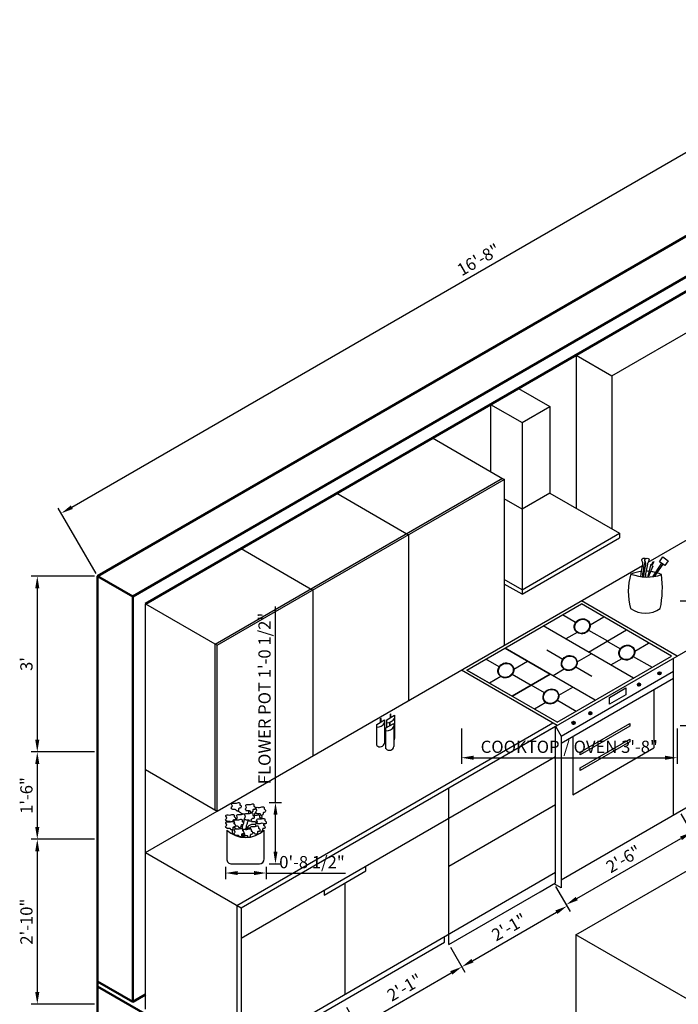
# Model space of a CAD drawing. Units: inches. Extents: x 5770 to 11891, y 3254 to 6808.
# Tile 2 of 15: x 5770 to 5905, y 3361 to 3563. Entities that reach past the tile are written whole.
import ezdxf

# ---------------------------------------------------------------- set-up
doc = ezdxf.new("R2010")
doc.units = ezdxf.units.IN
for name, color, linetype, lineweight in [('A-ANNO-DIMS', 2, 'Continuous', 18), ('A-ANNO-SYMB', 7, 'Continuous', 18), ('A-EQPM', 6, 'Continuous', 25), ('A-FURN', 8, 'Continuous', 25), ('A-WALL', 7, 'Continuous', 50)]:
    doc.layers.add(name, color=color, linetype=linetype, lineweight=lineweight)
doc.styles.get("Standard").update_dxf_attribs({"font": 'arial.ttf'})
doc.dimstyles.new('ISO-25', dxfattribs={"dimtxt": 2.5, "dimasz": 2.5, "dimexe": 1.25, "dimexo": 0.625, "dimtad": 1, "dimdec": 0, "dimlunit": 3, "dimtxsty": 'Standard', "dimcen": 2.5, "dimadec": 0, "dimazin": 0, "dimtfac": 1, "dimtdec": 0, "dimtmove": 0, "dimatfit": 3, "dimfxl": 1, "dimarcsym": 0})

# ---------------------------------------------------------------- blocks, each defined once
blk = doc.blocks.new('*D2')
at = {"layer": 'A-ANNO-DIMS', "color": 0, "lineweight": -2, "transparency": 16777216}
for p, q in [((5858.42, 3372.87), (5861.37, 3367.75)), ((5841.62, 3357.79), (5858.58, 3367.59)), ((5837.13, 3360.58), (5840.08, 3355.46))]:
    blk.add_line(p, q, dxfattribs=at)
at = {"layer": 'A-ANNO-DIMS', "color": 0, "transparency": 16777216}
for points in [[(5858.37, 3367.95), (5858.79, 3367.23), (5860.75, 3368.84)], [(5841.41, 3358.15), (5841.83, 3357.43), (5839.46, 3356.54)]]:
    blk.add_solid(points, dxfattribs=at)
at = {"layer": 'Defpoints', "color": 0, "transparency": 16777216}
for p in [(5858.1, 3373.41), (5860.75, 3368.84), (5836.81, 3361.12)]:
    blk.add_point(p, dxfattribs=at)
at = {"layer": 'A-ANNO-DIMS', "color": 0, "transparency": 16777216, "insert": (5849.16, 3364.32), "char_height": 2.5, "attachment_point": 5, "rotation": 30}
blk.add_mtext('2\'-1"', dxfattribs=at)
blk = doc.blocks.new('*D3')
at = {"layer": 'A-ANNO-DIMS', "color": 0, "lineweight": -2, "transparency": 16777216}
for p, q in [((5879.96, 3385.31), (5882.91, 3380.19)), ((5862.91, 3370.09), (5880.12, 3380.02)), ((5858.42, 3372.87), (5861.37, 3367.75))]:
    blk.add_line(p, q, dxfattribs=at)
at = {"layer": 'A-ANNO-DIMS', "color": 0, "transparency": 16777216}
for points in [[(5879.91, 3380.38), (5880.33, 3379.66), (5882.29, 3381.27)], [(5862.7, 3370.45), (5863.12, 3369.73), (5860.75, 3368.84)]]:
    blk.add_solid(points, dxfattribs=at)
at = {"layer": 'Defpoints', "color": 0, "transparency": 16777216}
for p in [(5879.65, 3385.85), (5882.29, 3381.27), (5858.1, 3373.41)]:
    blk.add_point(p, dxfattribs=at)
at = {"layer": 'A-ANNO-DIMS', "color": 0, "transparency": 16777216, "insert": (5870.58, 3376.68), "char_height": 2.5, "attachment_point": 5, "rotation": 30}
blk.add_mtext('2\'-1"', dxfattribs=at)
blk = doc.blocks.new('*D4')
at = {"layer": 'A-ANNO-DIMS', "color": 0, "lineweight": -2, "transparency": 16777216}
for p, q in [((5905.64, 3400.14), (5908.43, 3395.3)), ((5884.29, 3382.81), (5905.64, 3395.14)), ((5879.96, 3385.31), (5882.75, 3380.47))]:
    blk.add_line(p, q, dxfattribs=at)
at = {"layer": 'A-ANNO-DIMS', "color": 0, "transparency": 16777216}
for points in [[(5905.43, 3395.5), (5905.85, 3394.77), (5907.81, 3396.39)], [(5884.08, 3383.17), (5884.5, 3382.45), (5882.12, 3381.56)]]:
    blk.add_solid(points, dxfattribs=at)
at = {"layer": 'Defpoints', "color": 0, "transparency": 16777216}
for p in [(5905.33, 3400.68), (5907.81, 3396.39), (5879.65, 3385.85)]:
    blk.add_point(p, dxfattribs=at)
at = {"layer": 'A-ANNO-DIMS', "color": 0, "transparency": 16777216, "insert": (5894.02, 3390.62), "char_height": 2.5, "attachment_point": 5, "rotation": 30}
blk.add_mtext('2\'-6"', dxfattribs=at)
blk = doc.blocks.new('*D5')
at = {"layer": 'A-ANNO-DIMS', "color": 0, "lineweight": -2, "transparency": 16777216}
for p, q in [((5959, 3549.37), (5951.25, 3562.79)), ((5780.84, 3462.96), (5949.71, 3560.46)), ((5785.8, 3449.37), (5778.05, 3462.79))]:
    blk.add_line(p, q, dxfattribs=at)
at = {"layer": 'A-ANNO-DIMS', "color": 0, "transparency": 16777216}
for points in [[(5949.5, 3560.82), (5949.92, 3560.1), (5951.88, 3561.71)], [(5780.63, 3463.32), (5781.05, 3462.6), (5778.67, 3461.71)]]:
    blk.add_solid(points, dxfattribs=at)
at = {"layer": 'Defpoints', "color": 0, "transparency": 16777216}
for p in [(5951.88, 3561.71), (5959.31, 3548.83), (5786.11, 3448.83)]:
    blk.add_point(p, dxfattribs=at)
at = {"layer": 'A-ANNO-DIMS', "color": 0, "transparency": 16777216, "insert": (5864.32, 3513.36), "char_height": 2.5, "attachment_point": 5, "rotation": 30}
blk.add_mtext('16\'-8"', dxfattribs=at)
blk = doc.blocks.new('STOVE')
for p, q in [((5858.32, 3427.6), (5881.78, 3441.15)), ((5901.39, 3430.48), (5881.78, 3441.8)), ((5900.26, 3430.48), (5881.78, 3441.15)), ((5880.59, 3437.32), (5877.87, 3438.89)), ((5883.56, 3436.84), (5886.4, 3438.48)), ((5892.44, 3425.97), (5873.96, 3436.63)), ((5880.89, 3435.3), (5878.58, 3433.97)), ((5883.2, 3431.3), (5891.02, 3435.82)), ((5883.26, 3435.78), (5887.11, 3433.56)), ((5858.32, 3427.6), (5866.14, 3432.12)), ((5884.62, 3421.45), (5866.14, 3432.12)), ((5866.14, 3432.12), (5875.38, 3426.78)), ((5889.74, 3431.94), (5887.02, 3433.51)), ((5892.71, 3431.45), (5895.55, 3433.1)), ((5864.95, 3428.29), (5862.23, 3429.86)), ((5877.94, 3429.8), (5874.67, 3431.71)), ((5876.8, 3416.94), (5900.26, 3430.48)), ((5880.91, 3429.31), (5883.76, 3430.96)), ((5890.04, 3429.91), (5887.73, 3428.58)), ((5892.41, 3430.4), (5896.26, 3428.17)), ((5867.91, 3427.81), (5870.76, 3429.45)), ((5880.62, 3428.25), (5883.89, 3426.36)), ((5876.8, 3416.28), (5857.19, 3427.6)), ((5876.8, 3416.94), (5858.32, 3427.6)), ((5858.32, 3427.6), (5867.56, 3422.27)), ((5865.25, 3426.27), (5862.94, 3424.94)), ((5867.56, 3422.27), (5875.38, 3426.78)), ((5875.38, 3426.78), (5867.56, 3422.27)), ((5867.62, 3426.75), (5871.47, 3424.53)), ((5878.25, 3427.77), (5875.96, 3426.45)), ((5897.66, 3426.89), (5897.47, 3426.78)), ((5897.61, 3427.24), (5897.71, 3427.04)), ((5897.81, 3426.84), (5897.91, 3426.64)), ((5898.05, 3427.11), (5897.86, 3427)), ((5874.19, 3422.96), (5871.47, 3424.53)), ((5877.15, 3422.47), (5880, 3424.12)), ((5887.56, 3422.02), (5890.9, 3423.95)), ((5890.9, 3423.95), (5890.9, 3422.52)), ((5893.47, 3424.58), (5893.28, 3424.47)), ((5893.42, 3424.94), (5893.52, 3424.74)), ((5893.62, 3424.54), (5893.72, 3424.34)), ((5893.86, 3424.81), (5893.67, 3424.7)), ((5890.9, 3422.52), (5887.56, 3420.59)), ((5887.56, 3420.59), (5887.56, 3422.02)), ((5874.49, 3420.94), (5872.18, 3419.6)), ((5876.86, 3421.42), (5880.71, 3419.19)), ((5883.5, 3418.71), (5883.31, 3418.6)), ((5883.45, 3419.07), (5883.55, 3418.87)), ((5883.65, 3418.67), (5883.75, 3418.47)), ((5883.89, 3418.94), (5883.7, 3418.83)), ((5880.07, 3416.73), (5879.88, 3416.62)), ((5880.02, 3417.08), (5880.11, 3416.89)), ((5880.22, 3416.68), (5880.31, 3416.49)), ((5880.45, 3416.95), (5880.26, 3416.84))]:
    blk.add_line(p, q)
for centre, radius in [((5897.76, 3426.94), 0.335), ((5897.76, 3426.94), 0.114), ((5893.57, 3424.64), 0.335), ((5893.57, 3424.64), 0.114), ((5883.6, 3418.77), 0.335), ((5883.6, 3418.77), 0.114), ((5880.17, 3416.79), 0.335), ((5880.17, 3416.79), 0.114)]:
    blk.add_circle(centre, radius)
for centre in [(5881.94, 3436.57), (5891.09, 3431.18), (5879.29, 3429.04), (5866.29, 3427.54), (5875.53, 3422.2)]:
    blk.add_ellipse(centre, major_axis=(1.44, 0.83), ratio=0.905886, start_param=-3.141592653589793, end_param=3.141592653589793)
for points in [[(5880.58, 3435.79), (5880.67, 3435.64), (5880.78, 3435.52), (5881.13, 3435.25), (5881.41, 3435.14), (5882, 3435.11), (5882.31, 3435.18), (5882.86, 3435.47), (5883.09, 3435.69), (5883.4, 3436.21), (5883.48, 3436.51), (5883.44, 3437.08), (5883.32, 3437.35), (5882.95, 3437.77), (5882.7, 3437.91), (5882.13, 3438.04), (5881.82, 3438.02), (5881.24, 3437.82), (5880.98, 3437.64), (5880.59, 3437.18), (5880.47, 3436.91), (5880.39, 3436.33), (5880.44, 3436.03), (5880.58, 3435.79)], [(5889.73, 3430.4), (5889.82, 3430.26), (5889.93, 3430.13), (5890.28, 3429.86), (5890.56, 3429.76), (5891.15, 3429.72), (5891.46, 3429.79), (5892.01, 3430.08), (5892.24, 3430.3), (5892.55, 3430.82), (5892.63, 3431.13), (5892.59, 3431.7), (5892.47, 3431.97), (5892.1, 3432.38), (5891.85, 3432.53), (5891.28, 3432.65), (5890.96, 3432.63), (5890.39, 3432.43), (5890.13, 3432.25), (5889.74, 3431.8), (5889.61, 3431.52), (5889.53, 3430.95), (5889.59, 3430.65), (5889.73, 3430.4)], [(5877.94, 3428.26), (5878.02, 3428.12), (5878.13, 3427.99), (5878.49, 3427.72), (5878.76, 3427.62), (5879.36, 3427.58), (5879.67, 3427.65), (5880.21, 3427.94), (5880.45, 3428.16), (5880.76, 3428.68), (5880.83, 3428.98), (5880.79, 3429.56), (5880.68, 3429.83), (5880.3, 3430.24), (5880.05, 3430.39), (5879.48, 3430.51), (5879.17, 3430.49), (5878.6, 3430.29), (5878.33, 3430.11), (5877.95, 3429.66), (5877.82, 3429.38), (5877.74, 3428.81), (5877.8, 3428.51), (5877.94, 3428.26)], [(5864.94, 3426.76), (5865.03, 3426.61), (5865.14, 3426.48), (5865.49, 3426.21), (5865.77, 3426.11), (5866.36, 3426.08), (5866.67, 3426.15), (5867.22, 3426.44), (5867.45, 3426.66), (5867.76, 3427.18), (5867.83, 3427.48), (5867.79, 3428.05), (5867.68, 3428.32), (5867.31, 3428.73), (5867.05, 3428.88), (5866.49, 3429.01), (5866.17, 3428.99), (5865.6, 3428.79), (5865.34, 3428.61), (5864.95, 3428.15), (5864.82, 3427.88), (5864.74, 3427.3), (5864.8, 3427), (5864.94, 3426.76)], [(5874.18, 3421.42), (5874.26, 3421.28), (5874.38, 3421.15), (5874.73, 3420.88), (5875.01, 3420.78), (5875.6, 3420.74), (5875.91, 3420.81), (5876.46, 3421.1), (5876.69, 3421.32), (5877, 3421.85), (5877.07, 3422.15), (5877.03, 3422.72), (5876.92, 3422.99), (5876.55, 3423.4), (5876.29, 3423.55), (5875.72, 3423.67), (5875.41, 3423.66), (5874.84, 3423.45), (5874.58, 3423.27), (5874.19, 3422.82), (5874.06, 3422.54), (5873.98, 3421.97), (5874.04, 3421.67), (5874.18, 3421.42)]]:
    blk.add_open_spline(points, degree=3, knots=[-3.141593, -3.141593, -3.141593, -3.141593, -2.783595, -2.783595, -2.200125, -2.200125, -1.60877, -1.60877, -1.017506, -1.017506, -0.415089, -0.415089, 0.188805, 0.188805, 0.777819, 0.777819, 1.36577, 1.36577, 1.944973, 1.944973, 2.52628, 2.52628, 3.141593, 3.141593, 3.141593, 3.141593])
for p in [(5892.44, 3425.97), (5884.62, 3421.45)]:
    blk.add_point(p)
blk = doc.blocks.new('POT')
for p, q in [((5821.11, 3405.34), (5821.12, 3399.42)), ((5828.79, 3399.43), (5828.78, 3405.35)), ((5822.13, 3398.42), (5827.79, 3398.43))]:
    blk.add_line(p, q)
for centre, radius, start, end in [((5824.94, 3409.41), 5.59, 226.7933, 313.4113), ((5822.12, 3399.42), 1, 180.1023, 270.1023), ((5827.79, 3399.43), 1, 270.1023, 0.1023)]:
    blk.add_arc(centre, radius, start, end)
for points, knots in [([(5822.14, 3409.63), (5822.15, 3409.62), (5822.28, 3409.58), (5821.84, 3409.99), (5822.48, 3410.19), (5822.01, 3410.53), (5822.19, 3410.9), (5822.62, 3410.83), (5823.05, 3410.84), (5823.41, 3410.98), (5823.76, 3410.96), (5823.82, 3410.71), (5823.71, 3410.48), (5824, 3410.41), (5824.11, 3410.12), (5823.95, 3409.76), (5823.66, 3409.88), (5823.52, 3409.69), (5823.55, 3409.52), (5823.56, 3409.23), (5823.06, 3409.14), (5823.08, 3409.48), (5822.78, 3409.55), (5822.51, 3409.48), (5822.29, 3409.58), (5822.2, 3409.61), (5822.18, 3409.62)], [0, 0, 0, 0, 0.039437, 0.360257, 0.726322, 1.180919, 1.384496, 1.772178, 2.297526, 2.727606, 2.928942, 3.220339, 3.362126, 3.556196, 3.889983, 4.19796, 4.46721, 4.61651, 4.779686, 4.992372, 5.404712, 5.589005, 5.803395, 6.188281, 6.420646, 6.490513, 6.490513, 6.490513, 6.490513]), ([(5825.04, 3409.36), (5825.05, 3409.35), (5825.18, 3409.31), (5824.74, 3409.72), (5825.38, 3409.92), (5824.91, 3410.26), (5825.09, 3410.63), (5825.52, 3410.56), (5825.95, 3410.57), (5826.31, 3410.71), (5826.65, 3410.7), (5826.72, 3410.44), (5826.61, 3410.21), (5826.9, 3410.14), (5827.01, 3409.86), (5826.85, 3409.49), (5826.56, 3409.61), (5826.42, 3409.43), (5826.45, 3409.25), (5826.46, 3408.97), (5825.96, 3408.87), (5825.98, 3409.22), (5825.68, 3409.28), (5825.41, 3409.22), (5825.19, 3409.31), (5825.1, 3409.34), (5825.08, 3409.35)], [0, 0, 0, 0, 0.039437, 0.360257, 0.726322, 1.180919, 1.384496, 1.772178, 2.297526, 2.727606, 2.928942, 3.220339, 3.362126, 3.556196, 3.889983, 4.19796, 4.46721, 4.61651, 4.779686, 4.992372, 5.404712, 5.589005, 5.803395, 6.188281, 6.420646, 6.490513, 6.490513, 6.490513, 6.490513]), ([(5827.13, 3408.76), (5827.14, 3408.76), (5827.27, 3408.72), (5826.83, 3409.13), (5827.47, 3409.32), (5827, 3409.66), (5827.18, 3410.04), (5827.61, 3409.97), (5828.05, 3409.98), (5828.4, 3410.12), (5828.75, 3410.1), (5828.81, 3409.84), (5828.71, 3409.62), (5829, 3409.55), (5829.1, 3409.26), (5828.95, 3408.9), (5828.65, 3409.01), (5828.52, 3408.83), (5828.55, 3408.66), (5828.55, 3408.37), (5828.06, 3408.28), (5828.07, 3408.62), (5827.77, 3408.69), (5827.5, 3408.62), (5827.29, 3408.71), (5827.19, 3408.74), (5827.17, 3408.75)], [0, 0, 0, 0, 0.039437, 0.360257, 0.726322, 1.180919, 1.384496, 1.772178, 2.297526, 2.727606, 2.928942, 3.220339, 3.362126, 3.556196, 3.889983, 4.19796, 4.46721, 4.61651, 4.779686, 4.992372, 5.404712, 5.589005, 5.803395, 6.188281, 6.420646, 6.490513, 6.490513, 6.490513, 6.490513]), ([(5820.97, 3407.2), (5820.99, 3407.19), (5821.11, 3407.15), (5820.68, 3407.57), (5821.32, 3407.76), (5820.84, 3408.1), (5821.02, 3408.47), (5821.45, 3408.41), (5821.89, 3408.41), (5822.25, 3408.56), (5822.59, 3408.54), (5822.65, 3408.28), (5822.55, 3408.05), (5822.84, 3407.99), (5822.93, 3407.72), (5822.86, 3407.5), (5822.8, 3407.45)], [0, 0, 0, 0, 0.039437, 0.360257, 0.726322, 1.180919, 1.384496, 1.772178, 2.297526, 2.727606, 2.928942, 3.220339, 3.362126, 3.556196, 3.889983, 4.122088, 4.122088, 4.122088, 4.122088]), ([(5823.16, 3407.43), (5823.13, 3407.48), (5823, 3407.7), (5823.53, 3407.86), (5823.05, 3408.2), (5823.24, 3408.57), (5823.67, 3408.5), (5824.1, 3408.51), (5824.46, 3408.65), (5824.72, 3408.64), (5824.78, 3408.58), (5824.79, 3408.56)], [0.241721, 0.241721, 0.241721, 0.241721, 0.360257, 0.726322, 1.180919, 1.384496, 1.772178, 2.297526, 2.727606, 2.928942, 2.995165, 2.995165, 2.995165, 2.995165]), ([(5823.38, 3409.23), (5823.62, 3409.12), (5823.98, 3408.94), (5824.31, 3408.64), (5824.43, 3408.62)], [0, 0, 0, 0, 0.818095, 1.213546, 1.213546, 1.213546, 1.213546]), ([(5824.83, 3407.49), (5824.84, 3407.49), (5824.97, 3407.45), (5824.53, 3407.86), (5825.18, 3408.05), (5824.7, 3408.39), (5824.88, 3408.77), (5825.31, 3408.7), (5825.75, 3408.71), (5826.11, 3408.85), (5826.45, 3408.83), (5826.51, 3408.57), (5826.41, 3408.35), (5826.7, 3408.28), (5826.8, 3407.99), (5826.65, 3407.63), (5826.38, 3407.73), (5826.29, 3407.65), (5826.27, 3407.63)], [0, 0, 0, 0, 0.039437, 0.360257, 0.726322, 1.180919, 1.384496, 1.772178, 2.297526, 2.727606, 2.928942, 3.220339, 3.362126, 3.556196, 3.889983, 4.19796, 4.46721, 4.546762, 4.546762, 4.546762, 4.546762]), ([(5825.66, 3409.26), (5825.63, 3409.19), (5825.6, 3409.09), (5825.55, 3408.91), (5825.57, 3408.79), (5825.59, 3408.71)], [0, 0, 0, 0, 0.2062103, 0.3305427, 0.5571875, 0.5571875, 0.5571875, 0.5571875]), ([(5826.19, 3407.11), (5826.21, 3407.11), (5826.34, 3407.07), (5825.92, 3407.46), (5826.25, 3407.59), (5826.31, 3407.66)], [0, 0, 0, 0, 0.0394372, 0.3602568, 0.693565, 0.693565, 0.693565, 0.693565]), ([(5826.47, 3408.35), (5826.52, 3408.35), (5826.76, 3408.32), (5827.11, 3408.33), (5827.47, 3408.47), (5827.81, 3408.45), (5827.88, 3408.19), (5827.77, 3407.97), (5828.05, 3407.9), (5828.12, 3407.74), (5828.12, 3407.63)], [1.639371, 1.639371, 1.639371, 1.639371, 1.772178, 2.297526, 2.727606, 2.928942, 3.220339, 3.362126, 3.556196, 3.860816, 3.860816, 3.860816, 3.860816]), ([(5827.13, 3408.76), (5826.99, 3408.79), (5826.75, 3408.83), (5826.79, 3408.56), (5826.78, 3408.43), (5826.75, 3408.37), (5826.72, 3408.33)], [0, 0, 0, 0, 0.3286711, 0.5656891, 0.6105437, 0.7489262, 0.7489262, 0.7489262, 0.7489262]), ([(5827.18, 3406.68), (5827.16, 3406.82), (5827.62, 3406.96), (5827.15, 3407.3), (5827.33, 3407.67), (5827.76, 3407.6), (5828.2, 3407.61), (5828.55, 3407.75), (5828.9, 3407.73), (5828.96, 3407.48), (5828.85, 3407.25), (5829.15, 3407.18), (5829.25, 3406.89), (5829.1, 3406.53), (5828.8, 3406.65), (5828.67, 3406.47), (5828.68, 3406.36), (5828.69, 3406.29), (5828.69, 3406.29)], [0.36156, 0.36156, 0.36156, 0.36156, 0.726322, 1.180919, 1.384496, 1.772178, 2.297526, 2.727606, 2.928942, 3.220339, 3.362126, 3.556196, 3.889983, 4.19796, 4.46721, 4.61651, 4.779686, 4.795694, 4.795694, 4.795694, 4.795694]), ([(5828.24, 3408.34), (5828.24, 3408.26), (5828.25, 3408.15), (5828.29, 3407.98), (5828.23, 3407.83), (5828.22, 3407.71), (5828.22, 3407.65)], [0, 0, 0, 0, 0.243019, 0.3523221, 0.5049138, 0.7052748, 0.7052748, 0.7052748, 0.7052748]), ([(5820.97, 3405.77), (5820.98, 3405.77), (5821.11, 3405.73), (5820.67, 3406.14), (5821.31, 3406.33), (5820.83, 3406.67), (5821.02, 3407.05), (5821.45, 3406.98), (5821.88, 3406.99), (5822.24, 3407.13), (5822.58, 3407.11), (5822.65, 3406.85), (5822.54, 3406.63), (5822.83, 3406.56), (5822.94, 3406.27), (5822.78, 3405.91), (5822.49, 3406.02), (5822.35, 3405.84), (5822.38, 3405.67), (5822.39, 3405.38), (5821.89, 3405.29), (5821.91, 3405.63), (5821.6, 3405.7), (5821.34, 3405.63), (5821.12, 3405.72), (5821.03, 3405.75), (5821, 3405.76)], [0, 0, 0, 0, 0.039437, 0.360257, 0.726322, 1.180919, 1.384496, 1.772178, 2.297526, 2.727606, 2.928942, 3.220339, 3.362126, 3.556196, 3.889983, 4.19796, 4.46721, 4.61651, 4.779686, 4.992372, 5.404712, 5.589005, 5.803395, 6.188281, 6.420646, 6.490513, 6.490513, 6.490513, 6.490513]), ([(5821.88, 3407.02), (5821.88, 3407.02), (5821.84, 3407.07), (5821.61, 3407.12), (5821.35, 3407.06), (5821.13, 3407.15), (5821.03, 3407.18), (5821.01, 3407.19)], [5.588758, 5.588758, 5.588758, 5.588758, 5.5890049, 5.803395, 6.1882813, 6.4206461, 6.4905127, 6.4905127, 6.4905127, 6.4905127]), ([(5822.67, 3407.4), (5822.6, 3407.4), (5822.48, 3407.43), (5822.36, 3407.27), (5822.38, 3407.17), (5822.38, 3407.12)], [4.2739594, 4.2739594, 4.2739594, 4.2739594, 4.4672103, 4.6165101, 4.7723076, 4.7723076, 4.7723076, 4.7723076]), ([(5822.51, 3405.97), (5822.54, 3405.94), (5822.76, 3405.75), (5823.03, 3405.64), (5823.27, 3405.56)], [1.0148187, 1.0148187, 1.0148187, 1.0148187, 1.1544682, 1.8865276, 1.8865276, 1.8865276, 1.8865276]), ([(5822.6, 3406.64), (5822.65, 3406.69), (5822.9, 3406.83), (5822.49, 3407.12), (5822.68, 3407.49), (5823.11, 3407.42), (5823.54, 3407.43), (5823.9, 3407.57), (5824.24, 3407.55), (5824.31, 3407.29), (5824.2, 3407.07), (5824.49, 3407), (5824.6, 3406.71), (5824.44, 3406.35), (5824.15, 3406.47), (5824.01, 3406.28), (5824.04, 3406.11), (5824.05, 3405.82), (5823.55, 3405.73), (5823.57, 3406.07), (5823.26, 3406.14), (5823.05, 3406.08), (5822.89, 3406.12), (5822.86, 3406.13)], [0.516718, 0.516718, 0.516718, 0.516718, 0.726322, 1.180919, 1.384496, 1.772178, 2.297526, 2.727606, 2.928942, 3.220339, 3.362126, 3.556196, 3.889983, 4.19796, 4.46721, 4.61651, 4.779686, 4.992372, 5.404712, 5.589005, 5.803395, 6.188281, 6.278847, 6.278847, 6.278847, 6.278847]), ([(5822.7, 3404.34), (5822.71, 3404.33), (5822.84, 3404.29), (5822.4, 3404.71), (5823.04, 3404.9), (5822.57, 3405.24), (5822.75, 3405.61), (5823.18, 3405.55), (5823.62, 3405.55), (5823.97, 3405.7), (5824.32, 3405.68), (5824.38, 3405.42), (5824.27, 3405.19), (5824.43, 3405.16), (5824.5, 3405.11), (5824.5, 3405.11)], [0, 0, 0, 0, 0.039437, 0.360257, 0.726322, 1.180919, 1.384496, 1.772178, 2.297526, 2.727606, 2.928942, 3.220339, 3.362126, 3.556196, 3.579852, 3.579852, 3.579852, 3.579852]), ([(5824.33, 3406.42), (5824.29, 3406.13), (5824.22, 3405.69), (5824.56, 3405), (5824.96, 3404.05), (5824.43, 3403.93), (5824.32, 3403.9)], [0, 0, 0, 0, 0.812185, 1.274244, 2.451284, 2.763737, 2.763737, 2.763737, 2.763737]), ([(5824.89, 3407.5), (5824.82, 3407.5), (5824.69, 3407.53), (5824.57, 3407.37), (5824.6, 3407.19), (5824.61, 3407.02), (5824.52, 3406.95), (5824.49, 3406.93)], [4.2721359, 4.2721359, 4.2721359, 4.2721359, 4.4672103, 4.6165101, 4.7796861, 4.9923719, 5.082884, 5.082884, 5.082884, 5.082884]), ([(5825.5, 3407.39), (5825.43, 3407.26), (5825.32, 3407.03), (5825.28, 3406.61), (5825.03, 3406.18), (5825.09, 3405.65), (5824.85, 3405.5), (5824.83, 3405.49)], [0, 0, 0, 0, 0.447586, 0.762872, 1.22978, 1.947854, 2.042001, 2.042001, 2.042001, 2.042001]), ([(5826.98, 3406.47), (5826.77, 3406.49), (5826.35, 3406.54), (5825.78, 3406.31), (5825.33, 3405.99), (5825.07, 3405.66), (5824.88, 3405.53), (5824.83, 3405.49)], [0, 0, 0, 0, 0.620136, 1.244128, 1.783255, 2.276688, 2.482027, 2.482027, 2.482027, 2.482027]), ([(5825.94, 3405.79), (5825.86, 3405.78), (5825.66, 3405.76), (5825.35, 3405.68), (5825.08, 3405.53), (5824.89, 3405.5), (5824.83, 3405.49)], [0, 0, 0, 0, 0.242701, 0.588723, 0.956, 1.159466, 1.159466, 1.159466, 1.159466]), ([(5826.21, 3407.19), (5826.21, 3407.19), (5826.12, 3407.08), (5825.76, 3407.01), (5825.78, 3407.35), (5825.47, 3407.42), (5825.21, 3407.35), (5824.99, 3407.44), (5824.89, 3407.47), (5824.87, 3407.48)], [4.988606, 4.988606, 4.988606, 4.988606, 4.992372, 5.404712, 5.589005, 5.803395, 6.188281, 6.420646, 6.490513, 6.490513, 6.490513, 6.490513]), ([(5826.08, 3405.55), (5826.03, 3405.64), (5825.87, 3405.8), (5826.03, 3406.12), (5826.46, 3406.05), (5826.9, 3406.06), (5827.25, 3406.2), (5827.6, 3406.18), (5827.66, 3405.92), (5827.55, 3405.7), (5827.84, 3405.63), (5827.95, 3405.34), (5827.8, 3404.98), (5827.5, 3405.09), (5827.36, 3404.91), (5827.4, 3404.74), (5827.4, 3404.45), (5826.9, 3404.36), (5826.92, 3404.7), (5826.67, 3404.76), (5826.51, 3404.73), (5826.43, 3404.73)], [0.890699, 0.890699, 0.890699, 0.890699, 1.180919, 1.384496, 1.772178, 2.297526, 2.727606, 2.928942, 3.220339, 3.362126, 3.556196, 3.889983, 4.19796, 4.46721, 4.61651, 4.779686, 4.992372, 5.404712, 5.589005, 5.803395, 6.061557, 6.061557, 6.061557, 6.061557]), ([(5827.19, 3406.73), (5827.18, 3406.74), (5827.13, 3406.79), (5827.14, 3406.97), (5826.83, 3407.04), (5826.57, 3406.97), (5826.35, 3407.07), (5826.26, 3407.1), (5826.23, 3407.1)], [5.365177, 5.365177, 5.365177, 5.365177, 5.404712, 5.589005, 5.803395, 6.188281, 6.420646, 6.490513, 6.490513, 6.490513, 6.490513]), ([(5827.13, 3406.15), (5827.08, 3406.23), (5826.92, 3406.4), (5827.08, 3406.72), (5827.51, 3406.65), (5827.94, 3406.66), (5828.3, 3406.8), (5828.64, 3406.78), (5828.71, 3406.53), (5828.6, 3406.3), (5828.89, 3406.23), (5829, 3405.94), (5828.84, 3405.58), (5828.55, 3405.7), (5828.41, 3405.52), (5828.44, 3405.34), (5828.45, 3405.06), (5827.95, 3404.96), (5827.97, 3405.24), (5827.91, 3405.29), (5827.9, 3405.3)], [0.882232, 0.882232, 0.882232, 0.882232, 1.180919, 1.384496, 1.772178, 2.297526, 2.727606, 2.928942, 3.220339, 3.362126, 3.556196, 3.889983, 4.19796, 4.46721, 4.61651, 4.779686, 4.992372, 5.404712, 5.589005, 5.643787, 5.643787, 5.643787, 5.643787]), ([(5822.31, 3405.44), (5822.23, 3405.26), (5822.08, 3404.92), (5822.41, 3404.62), (5822.75, 3404.32), (5823.03, 3404.22), (5823.26, 3404.13)], [0, 0, 0, 0, 0.523026, 1.01073, 1.154468, 1.886528, 1.886528, 1.886528, 1.886528]), ([(5824.62, 3404.93), (5824.62, 3404.9), (5824.63, 3404.75), (5824.52, 3404.47), (5824.22, 3404.59), (5824.08, 3404.41), (5824.12, 3404.23), (5824.12, 3403.95), (5823.62, 3403.85), (5823.64, 3404.2), (5823.34, 3404.26), (5823.07, 3404.2), (5822.85, 3404.29), (5822.76, 3404.32), (5822.74, 3404.33)], [3.784791, 3.784791, 3.784791, 3.784791, 3.889983, 4.19796, 4.46721, 4.61651, 4.779686, 4.992372, 5.404712, 5.589005, 5.803395, 6.188281, 6.420646, 6.490513, 6.490513, 6.490513, 6.490513]), ([(5824.18, 3404.51), (5824.2, 3404.46), (5824.25, 3404.33), (5824.33, 3404.14), (5824.3, 3403.86), (5824.38, 3403.85), (5824.38, 3403.85)], [0, 0, 0, 0, 0.1514383, 0.4275376, 0.6941888, 0.6941902, 0.6941902, 0.6941902, 0.6941902]), ([(5824.88, 3404.14), (5824.82, 3404.09), (5824.73, 3404.01), (5824.52, 3404.01), (5824.48, 3403.83), (5824.4, 3403.85), (5824.38, 3403.85)], [0, 0, 0, 0, 0.2193464, 0.3741289, 0.5521828, 0.5973013, 0.5973013, 0.5973013, 0.5973013]), ([(5824.5, 3404.25), (5824.52, 3404.25), (5824.64, 3404.21), (5824.42, 3404.42), (5824.41, 3404.54), (5824.41, 3404.54)], [0, 0, 0, 0, 0.0394372, 0.3602568, 0.3665838, 0.3665838, 0.3665838, 0.3665838]), ([(5824.62, 3404.93), (5824.57, 3405.03), (5824.39, 3405.2), (5824.55, 3405.53), (5824.98, 3405.46), (5825.42, 3405.47), (5825.78, 3405.61), (5826.12, 3405.59), (5826.18, 3405.33), (5826.08, 3405.11), (5826.37, 3405.04), (5826.47, 3404.75), (5826.32, 3404.39), (5826.02, 3404.5), (5825.89, 3404.32), (5825.92, 3404.15), (5825.92, 3403.86), (5825.43, 3403.77), (5825.45, 3404.11), (5825.14, 3404.18), (5824.88, 3404.11), (5824.66, 3404.2), (5824.56, 3404.23), (5824.54, 3404.24)], [0.859859, 0.859859, 0.859859, 0.859859, 1.180919, 1.384496, 1.772178, 2.297526, 2.727606, 2.928942, 3.220339, 3.362126, 3.556196, 3.889983, 4.19796, 4.46721, 4.61651, 4.779686, 4.992372, 5.404712, 5.589005, 5.803395, 6.188281, 6.420646, 6.490513, 6.490513, 6.490513, 6.490513])]:
    blk.add_open_spline(points, degree=3, knots=knots)
blk = doc.blocks.new('*D20')
at = {"layer": 'A-ANNO-DIMS', "color": 0, "lineweight": -2, "transparency": 16777216}
for p, q in [((5785.48, 3448.83), (5772.51, 3448.83)), ((5773.76, 3446.33), (5773.76, 3415.35)), ((5785.48, 3412.85), (5772.51, 3412.85))]:
    blk.add_line(p, q, dxfattribs=at)
at = {"layer": 'A-ANNO-DIMS', "color": 0, "transparency": 16777216}
for points in [[(5773.34, 3446.33), (5774.18, 3446.33), (5773.76, 3448.83)], [(5773.34, 3415.35), (5774.18, 3415.35), (5773.76, 3412.85)]]:
    blk.add_solid(points, dxfattribs=at)
at = {"layer": 'Defpoints', "color": 0, "transparency": 16777216}
for p in [(5786.11, 3448.83), (5773.76, 3412.85), (5786.11, 3412.85)]:
    blk.add_point(p, dxfattribs=at)
at = {"layer": 'A-ANNO-DIMS', "color": 0, "transparency": 16777216, "insert": (5771.86, 3430.84), "char_height": 2.5, "attachment_point": 5, "rotation": 90}
blk.add_mtext("3'", dxfattribs=at)
blk = doc.blocks.new('*D21')
at = {"layer": 'A-ANNO-DIMS', "color": 0, "lineweight": -2, "transparency": 16777216}
for p, q in [((5785.48, 3412.85), (5772.51, 3412.85)), ((5773.76, 3410.35), (5773.76, 3397.47)), ((5785.48, 3394.97), (5772.51, 3394.97))]:
    blk.add_line(p, q, dxfattribs=at)
at = {"layer": 'A-ANNO-DIMS', "color": 0, "transparency": 16777216}
for points in [[(5773.34, 3410.35), (5774.18, 3410.35), (5773.76, 3412.85)], [(5773.34, 3397.47), (5774.18, 3397.47), (5773.76, 3394.97)]]:
    blk.add_solid(points, dxfattribs=at)
at = {"layer": 'Defpoints', "color": 0, "transparency": 16777216}
for p in [(5786.11, 3412.85), (5773.76, 3394.97), (5786.11, 3394.97)]:
    blk.add_point(p, dxfattribs=at)
at = {"layer": 'A-ANNO-DIMS', "color": 0, "transparency": 16777216, "insert": (5771.86, 3403.91), "char_height": 2.5, "attachment_point": 5, "rotation": 90}
blk.add_mtext('1\'-6"', dxfattribs=at)
blk = doc.blocks.new('*D22')
at = {"layer": 'A-ANNO-DIMS', "color": 0, "lineweight": -2, "transparency": 16777216}
for p, q in [((5785.48, 3394.97), (5772.51, 3394.97)), ((5773.76, 3392.47), (5773.76, 3363.69)), ((5785.48, 3361.19), (5772.51, 3361.19))]:
    blk.add_line(p, q, dxfattribs=at)
at = {"layer": 'A-ANNO-DIMS', "color": 0, "transparency": 16777216}
for points in [[(5773.34, 3392.47), (5774.18, 3392.47), (5773.76, 3394.97)], [(5773.34, 3363.69), (5774.18, 3363.69), (5773.76, 3361.19)]]:
    blk.add_solid(points, dxfattribs=at)
at = {"layer": 'Defpoints', "color": 0, "transparency": 16777216}
for p in [(5786.11, 3394.97), (5773.76, 3361.19), (5786.11, 3361.19)]:
    blk.add_point(p, dxfattribs=at)
at = {"layer": 'A-ANNO-DIMS', "color": 0, "transparency": 16777216, "insert": (5771.86, 3378.08), "char_height": 2.5, "attachment_point": 5, "rotation": 90}
blk.add_mtext('2\'-10"', dxfattribs=at)
blk = doc.blocks.new('*D30')
at = {"layer": 'A-ANNO-DIMS', "color": 0, "lineweight": -2, "transparency": 16777216}
for p, q in [((5860.65, 3417.65), (5860.65, 3410.4)), ((5904.85, 3417.65), (5904.85, 3410.4)), ((5863.15, 3411.65), (5902.35, 3411.65))]:
    blk.add_line(p, q, dxfattribs=at)
at = {"layer": 'A-ANNO-DIMS', "color": 0, "transparency": 16777216}
for points in [[(5863.15, 3412.07), (5863.15, 3411.23), (5860.65, 3411.65)], [(5902.35, 3412.07), (5902.35, 3411.23), (5904.85, 3411.65)]]:
    blk.add_solid(points, dxfattribs=at)
at = {"layer": 'Defpoints', "color": 0, "transparency": 16777216}
for p in [(5860.65, 3418.28), (5904.85, 3418.28), (5904.85, 3411.65)]:
    blk.add_point(p, dxfattribs=at)
at = {"layer": 'A-ANNO-DIMS', "color": 0, "transparency": 16777216, "insert": (5882.75, 3413.57), "char_height": 2.5, "attachment_point": 5}
blk.add_mtext('COOKTOP / OVEN 3\'-8"', dxfattribs=at)
blk = doc.blocks.new('*D31')
at = {"layer": 'A-ANNO-DIMS', "color": 0, "lineweight": -2, "transparency": 16777216}
for p, q in [((5905.48, 3443.8), (5912.73, 3443.8)), ((5911.48, 3420.78), (5911.48, 3441.3)), ((5905.48, 3418.28), (5912.73, 3418.28))]:
    blk.add_line(p, q, dxfattribs=at)
at = {"layer": 'A-ANNO-DIMS', "color": 0, "transparency": 16777216}
for points in [[(5911.07, 3441.3), (5911.9, 3441.3), (5911.48, 3443.8)], [(5911.07, 3420.78), (5911.9, 3420.78), (5911.48, 3418.28)]]:
    blk.add_solid(points, dxfattribs=at)
at = {"layer": 'Defpoints', "color": 0, "transparency": 16777216}
for p in [(5904.85, 3443.8), (5911.48, 3443.8), (5904.85, 3418.28)]:
    blk.add_point(p, dxfattribs=at)
at = {"layer": 'A-ANNO-DIMS', "color": 0, "transparency": 16777216, "insert": (5909.57, 3431.04), "char_height": 2.5, "attachment_point": 5, "rotation": 90}
blk.add_mtext('2\'-1 1/2"', dxfattribs=at)
blk = doc.blocks.new('*D42')
at = {"layer": 'A-ANNO-DIMS', "color": 0, "lineweight": -2, "transparency": 16777216}
for p, q in [((5822.56, 3402.47), (5822.56, 3442.61)), ((5821.3, 3402.47), (5823.81, 3402.47)), ((5822.56, 3392.42), (5822.56, 3399.97)), ((5821.3, 3389.92), (5823.81, 3389.92))]:
    blk.add_line(p, q, dxfattribs=at)
at = {"layer": 'A-ANNO-DIMS', "color": 0, "transparency": 16777216}
for points in [[(5822.15, 3399.97), (5822.98, 3399.97), (5822.56, 3402.47)], [(5822.15, 3392.42), (5822.98, 3392.42), (5822.56, 3389.92)]]:
    blk.add_solid(points, dxfattribs=at)
at = {"layer": 'Defpoints', "color": 0, "transparency": 16777216}
for p in [(5820.68, 3402.47), (5822.56, 3402.47), (5820.68, 3389.92)]:
    blk.add_point(p, dxfattribs=at)
at = {"layer": 'A-ANNO-DIMS', "color": 0, "transparency": 16777216, "insert": (5820.64, 3423.79), "char_height": 2.5, "attachment_point": 5, "rotation": 90}
blk.add_mtext('FLOWER POT 1\'-0 1/2"', dxfattribs=at)
blk = doc.blocks.new('*D43')
at = {"layer": 'A-ANNO-DIMS', "color": 0, "lineweight": -2, "transparency": 16777216}
for p, q in [((5812.32, 3389.3), (5812.32, 3386.79)), ((5814.82, 3388.04), (5818.18, 3388.04)), ((5820.68, 3389.3), (5820.68, 3386.79)), ((5820.68, 3388.04), (5836.9, 3388.04))]:
    blk.add_line(p, q, dxfattribs=at)
at = {"layer": 'A-ANNO-DIMS', "color": 0, "transparency": 16777216}
for points in [[(5814.82, 3388.45), (5814.82, 3387.62), (5812.32, 3388.04)], [(5818.18, 3388.45), (5818.18, 3387.62), (5820.68, 3388.04)]]:
    blk.add_solid(points, dxfattribs=at)
at = {"layer": 'Defpoints', "color": 0, "transparency": 16777216}
for p in [(5812.32, 3389.92), (5820.68, 3389.92), (5820.68, 3388.04)]:
    blk.add_point(p, dxfattribs=at)
at = {"layer": 'A-ANNO-DIMS', "color": 0, "transparency": 16777216, "insert": (5830.04, 3389.95), "char_height": 2.5, "attachment_point": 5}
blk.add_mtext('0\'-8 1/2"', dxfattribs=at)

msp = doc.modelspace()

# ---------------------------------------------------------------- linework, layer by layer
at = {"layer": 'A-ANNO-SYMB'}
for p in [(5869.44, 3468.64), (5840.03, 3451.66)]:
    msp.add_point(p, dxfattribs=at)
at = {"layer": 'A-FURN'}
for p, q in [((5891.5, 3489.87), (5918.64, 3505.53)), ((5884.15, 3494.11), (5891.5, 3489.87)), ((5884.15, 3494.11), (5884.15, 3462.76)), ((5891.5, 3489.87), (5891.5, 3458.51)), ((5872.32, 3487.28), (5878.77, 3483.55)), ((5866.63, 3483.99), (5873.08, 3480.27)), ((5866.63, 3483.99), (5866.63, 3470.27)), ((5873.08, 3480.27), (5878.77, 3483.55)), ((5878.77, 3483.55), (5878.77, 3465.86)), ((5873.08, 3480.27), (5873.08, 3462.58)), ((5854.74, 3477.13), (5869.44, 3468.64)), ((5884.15, 3477.13), (5884.15, 3462.76)), ((5810.21, 3434.91), (5869.04, 3468.88)), ((5810.62, 3434.68), (5869.44, 3468.64)), ((5869.44, 3468.64), (5869.44, 3434.68)), ((5835.13, 3465.81), (5849.84, 3457.32)), ((5873.08, 3462.58), (5869.44, 3464.68)), ((5878.77, 3465.86), (5873.08, 3462.58)), ((5878.77, 3465.86), (5893.07, 3457.61)), ((5873.08, 3462.58), (5873.08, 3445.12)), ((5898.94, 3451.71), (5918.64, 3463.08)), ((5849.84, 3457.32), (5849.84, 3423.36)), ((5873.08, 3446.06), (5893.07, 3457.61)), ((5873.08, 3445.12), (5893.07, 3456.66)), ((5893.07, 3457.61), (5893.07, 3456.66)), ((5815.52, 3454.49), (5830.23, 3446)), ((5901.21, 3451.79), (5901.9, 3452.78)), ((5901.9, 3452.78), (5903.04, 3451.98)), ((5810.62, 3400.72), (5897.76, 3451.02)), ((5898.83, 3448.65), (5899.52, 3451.31)), ((5899.87, 3450.9), (5898.88, 3448.65)), ((5899.52, 3451.31), (5899.67, 3451.23)), ((5899.67, 3451.23), (5899.97, 3451.83)), ((5899.76, 3451.18), (5899.67, 3451.01)), ((5899.67, 3451.01), (5899.87, 3450.9)), ((5900.06, 3451.79), (5899.76, 3451.18)), ((5901.65, 3451.49), (5899.77, 3448.72)), ((5899.97, 3451.83), (5900.06, 3451.79)), ((5901.89, 3451.32), (5900.16, 3448.77)), ((5902.34, 3451), (5901.21, 3451.79)), ((5903.04, 3451.98), (5902.34, 3451)), ((5873.08, 3446.06), (5869.44, 3448.16)), ((5830.23, 3446), (5830.23, 3412.04)), ((5873.08, 3445.12), (5869.44, 3447.22)), ((5815.52, 3380.9), (5925.99, 3444.68)), ((5795.91, 3409.21), (5795.91, 3443.17)), ((5795.91, 3443.17), (5810.62, 3434.68)), ((5810.21, 3400.95), (5810.21, 3434.91)), ((5810.62, 3400.72), (5810.62, 3434.68)), ((5904.11, 3399.98), (5904.11, 3432.05)), ((5881.06, 3416.07), (5904.11, 3429.38)), ((5881.06, 3414.64), (5904.11, 3427.95)), ((5900.08, 3425.62), (5900.08, 3413.67)), ((5884.12, 3375.37), (5967.26, 3423.37)), ((5845.34, 3419.4), (5846.96, 3420.34)), ((5846.22, 3420.61), (5846.05, 3420.51)), ((5846.05, 3420.51), (5846.05, 3419.81)), ((5846.22, 3419.91), (5846.22, 3420.61)), ((5846.96, 3420.34), (5846.96, 3415.58)), ((5814.66, 3381.4), (5879.39, 3418.78)), ((5815.52, 3380.9), (5879.96, 3418.11)), ((5843.3, 3418.48), (5844.92, 3419.41)), ((5843.3, 3414.17), (5843.3, 3418.48)), ((5844.18, 3419.69), (5844.01, 3419.59)), ((5844.01, 3419.59), (5844.01, 3418.89)), ((5844.18, 3418.99), (5844.18, 3419.69)), ((5844.92, 3419.41), (5844.92, 3414.66)), ((5845.2, 3417.75), (5846.83, 3418.69)), ((5845.2, 3413.45), (5845.2, 3417.75)), ((5845.34, 3417.83), (5845.34, 3419.4)), ((5846.09, 3418.96), (5845.92, 3418.86)), ((5845.92, 3418.86), (5845.92, 3418.16)), ((5846.09, 3418.27), (5846.09, 3418.96)), ((5846.83, 3418.69), (5846.83, 3413.94)), ((5879.96, 3386.03), (5879.96, 3418.11)), ((5879.96, 3418.11), (5881.06, 3416.07)), ((5885, 3412.77), (5895.17, 3418.65)), ((5895.17, 3418.1), (5885, 3412.22)), ((5895.17, 3418.65), (5895.17, 3418.1)), ((5881.06, 3416.07), (5881.06, 3385.03)), ((5883.47, 3416.03), (5883.47, 3404.08)), ((5885, 3409.61), (5895.17, 3415.48)), ((5895.17, 3414.93), (5885, 3409.06)), ((5895.17, 3415.48), (5895.17, 3414.93)), ((5815.52, 3374.71), (5879.96, 3411.91)), ((5883.47, 3404.08), (5900.08, 3413.67)), ((5885, 3412.22), (5885, 3412.77)), ((5881.06, 3386.67), (5923.86, 3411.38)), ((5795.91, 3392.22), (5795.91, 3409.21)), ((5795.91, 3409.21), (5810.62, 3400.72)), ((5885, 3409.06), (5885, 3409.61)), ((5858.1, 3373.41), (5858.1, 3405.49)), ((5858.1, 3389.45), (5879.96, 3402.07)), ((5795.91, 3392.22), (5810.62, 3400.72)), ((5795.91, 3360.15), (5795.91, 3392.22)), ((5795.91, 3392.22), (5815.52, 3380.9)), ((5879.96, 3388.14), (5815.52, 3350.85)), ((5832.54, 3383.52), (5841.08, 3388.46)), ((5841.08, 3388.46), (5841.08, 3389.47)), ((5836.81, 3363.17), (5836.81, 3385.99)), ((5876.8, 3384.21), (5879.96, 3386.03)), ((5881.06, 3385.03), (5879.65, 3385.85)), ((5832.54, 3384.53), (5832.54, 3383.52)), ((5858.1, 3373.41), (5876.8, 3384.21)), ((5814.66, 3381.4), (5814.66, 3349.33)), ((5815.52, 3380.9), (5815.52, 3350.85)), ((5814.66, 3349.33), (5857.18, 3373.88)), ((5857.18, 3373.88), (5857.18, 3374.95)), ((5920.5, 3354.37), (5884.12, 3375.37)), ((5884.12, 3375.37), (5884.12, 3345.37))]:
    msp.add_line(p, q, dxfattribs=at)
for centre, radius, start, end in [((5907.52, 3445.63), 12.68, 163.2653, 195.6988), ((5898.38, 3441.82), 8.03, 95.9776, 111.9225), ((5898.68, 3457.62), 8.97, 248.4575, 289.3976), ((5898.38, 3441.82), 8.03, 91.4862, 93.8684), ((5898.38, 3441.82), 8.03, 84.6642, 89.3253), ((5898.38, 3441.82), 8.03, 75.6613, 82.8218), ((5898.38, 3441.82), 8.03, 75.6613, 76.548), ((5898.38, 3441.82), 8.03, 65.9327, 73.4572), ((5879.79, 3446.49), 22.03, 348.7732, 6.9701), ((5898.36, 3446.61), 5.36, 235.4256, 304.5744), ((5843.38, 3419.74), 1.83, 267.5109, 327.8211), ((5845.28, 3419.01), 1.83, 267.5109, 327.8211), ((5845.42, 3420.66), 1.83, 267.5109, 327.8211), ((5843.98, 3414.85), 0.963, 224.9104, 348.6154), ((5845.89, 3414.13), 0.963, 224.9104, 348.6154), ((5846.02, 3415.77), 0.963, 327.5254, 348.6154)]:
    msp.add_arc(centre, radius, start, end, dxfattribs=at)
for points, knots in [([(5897.42, 3448.74), (5897.51, 3449.54), (5897.61, 3450.46), (5897.9, 3451.62), (5897.56, 3451.95), (5897.65, 3452.57), (5898.24, 3452.59), (5898.4, 3452.42)], [0.016818, 0.016818, 0.016818, 0.016818, 1.646284, 1.890088, 2.223298, 2.479698, 2.929344, 2.929344, 2.929344, 2.929344]), ([(5898.04, 3448.67), (5898.12, 3449.48), (5898.22, 3450.41), (5898.52, 3451.58), (5898.18, 3451.91), (5898.27, 3452.54), (5899.07, 3452.55), (5899.12, 3451.96), (5898.86, 3451.65), (5898.55, 3450.52), (5898.41, 3449.53), (5898.3, 3448.66)], [0, 0, 0, 0, 1.646284, 1.890088, 2.223298, 2.479698, 2.947513, 3.158169, 3.495076, 3.714111, 5.454719, 5.454719, 5.454719, 5.454719]), ([(5898.33, 3451.78), (5898.3, 3451.73), (5898.21, 3451.58), (5897.93, 3450.56), (5897.8, 3449.57), (5897.68, 3448.7)], [3.378802, 3.378802, 3.378802, 3.378802, 3.495076, 3.714111, 5.454719, 5.454719, 5.454719, 5.454719])]:
    msp.add_open_spline(points, degree=3, knots=knots, dxfattribs=at)
at = {"layer": 'A-WALL'}
for p, q in [((5959.31, 3548.83), (5786.11, 3448.83)), ((5795.91, 3446.17), (5959.31, 3540.51)), ((5795.91, 3443.17), (5959.31, 3537.51)), ((5786.11, 3448.83), (5786.11, 3364.83)), ((5793.32, 3444.67), (5786.11, 3448.83)), ((5795.91, 3446.17), (5793.32, 3444.67)), ((5793.32, 3361.65), (5793.32, 3444.67)), ((5793.32, 3361.65), (5786.11, 3365.81)), ((5962.44, 3263.03), (5786.11, 3364.83)), ((5786.11, 3364.83), (5786.11, 3355.83)), ((5793.32, 3361.65), (5795.91, 3363.15))]:
    msp.add_line(p, q, dxfattribs=at)

# ---------------------------------------------------------------- block references
at = {"layer": 'A-EQPM'}
msp.add_blockref('STOVE', (3.46, 2), dxfattribs=at)
at = {"layer": 'A-FURN'}
msp.add_blockref('POT', (-8.53, -8.5), dxfattribs=at)

# ---------------------------------------------------------------- dimensions: what is measured, and where the dimension line sits
at = {"layer": 'A-ANNO-DIMS'}
for p1, p2, distance, picture, middle in [((5786.11, 3448.83), (5959.31, 3548.83), 14.87, '*D5', (5864.32, 3513.36)), ((5786.11, 3448.83), (5786.11, 3412.85), -12.35, '*D20', (5771.86, 3430.84)), ((5786.11, 3412.85), (5786.11, 3394.97), -12.35, '*D21', (5771.86, 3403.91)), ((5879.65, 3385.85), (5905.33, 3400.68), -4.96, '*D4', (5894.02, 3390.62)), ((5786.11, 3394.97), (5786.11, 3361.19), -12.35, '*D22', (5771.86, 3378.08)), ((5858.1, 3373.41), (5879.65, 3385.85), -5.29, '*D3', (5870.58, 3376.68)), ((5836.81, 3361.12), (5858.1, 3373.41), -5.29, '*D2', (5849.16, 3364.32))]:
    dim = msp.add_aligned_dim(p1=p1, p2=p2, distance=distance, dimstyle='ISO-25', override={"dimclrd": 0, "dimclre": 0, "dimclrt": 0}, dxfattribs=at)
    dim.commit()
    dim.dimension.update_dxf_attribs({"geometry": picture, "text_midpoint": middle})
dim = msp.add_linear_dim(base=(5822.5621, 3402.4735), p1=(5820.6791, 3389.92), p2=(5820.6791, 3402.4735), angle=90, text='FLOWER POT <>', dimstyle='ISO-25', override={"dimdec": 1, "dimlfac": 1, "dimrnd": 0, "dimzin": 1, "dimdsep": 46, "dimlunit": 4, "dimfrac": 2}, dxfattribs=at)
dim.commit()
dim.dimension.update_dxf_attribs({"geometry": '*D42', "text_midpoint": (5820.6436, 3423.7934)})
dim = msp.add_linear_dim(base=(5911.48, 3443.8), p1=(5904.85, 3418.28), p2=(5904.85, 3443.8), angle=90, dimstyle='ISO-25', override={"dimdec": 1, "dimlfac": 1, "dimrnd": 0, "dimzin": 1, "dimdsep": 46, "dimlunit": 4, "dimfrac": 2}, dxfattribs=at)
dim.commit()
dim.dimension.update_dxf_attribs({"geometry": '*D31', "text_midpoint": (5909.57, 3431.04)})
dim = msp.add_linear_dim(base=(5904.85, 3411.65), p1=(5860.65, 3418.28), p2=(5904.85, 3418.28), text='COOKTOP / OVEN <>', dimstyle='ISO-25', override={"dimdec": 1, "dimlfac": 1, "dimrnd": 0, "dimzin": 1, "dimdsep": 46, "dimlunit": 4, "dimfrac": 2}, dxfattribs=at)
dim.commit()
dim.dimension.update_dxf_attribs({"geometry": '*D30', "text_midpoint": (5882.75, 3413.57)})
dim = msp.add_linear_dim(base=(5820.68, 3388.04), p1=(5812.32, 3389.92), p2=(5820.68, 3389.92), dimstyle='ISO-25', override={"dimdec": 1, "dimlfac": 1, "dimrnd": 0, "dimzin": 1, "dimdsep": 46, "dimlunit": 4, "dimfrac": 2}, dxfattribs=at)
dim.commit()
dim.dimension.update_dxf_attribs({"geometry": '*D43', "text_midpoint": (5830.04, 3389.95)})

doc.saveas('drawing.dxf')
